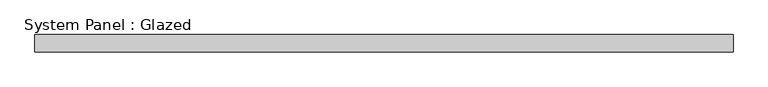
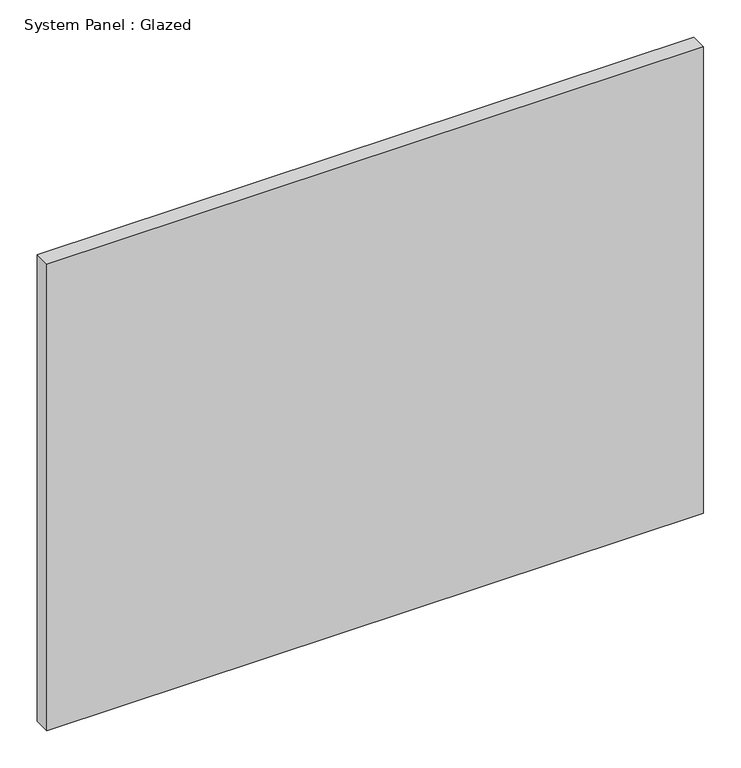
"""IFC4 building model written with IfcOpenShell, lengths in millimetres: plate geometry, System Panel : Glazed."""

from ifc_helpers import new_model, si_unit, origin, origin_with_axes, place, context, project, spatial, polyline, outline, extrude, source, transform, mapped, element, save


def system_panel_glazed_51d5fa28(model_context):
    return source(origin(), model_context, "Body", "SweptSolid", [
        extrude(outline(polyline([(508.92075, 19.05), (-508.92075, 19.05), (-508.92075, 44.45), (508.92075, 44.45), (508.92075, 19.05)])), origin_with_axes(), (0.0, 0.0, 1.0), 763.8415),
    ])


if __name__ == "__main__":
    model = new_model("IFC4")
    model_context = context("Model", 3, world=origin())
    ifc_project = project(units=[si_unit("LENGTHUNIT", "METRE", prefix="MILLI")], contexts=[model_context])
    site = spatial("IfcSite", under=ifc_project)
    building = spatial("IfcBuilding", under=site)
    placement = place(None, origin())
    system_panel_glazed_shape = system_panel_glazed_51d5fa28(model_context)
    element("IfcPlate", 1, ObjectType="System Panel : Glazed", at=placement, inside=building, context=model_context, shape_type="MappedRepresentation", body=[
        mapped(system_panel_glazed_shape, transform((0.0, 0.0, 0.0), x_axis=(1.0, 0.0, 0.0), y_axis=(0.0, 1.0, 0.0), z_axis=(0.0, 0.0, 1.0))),
    ])
    save(model, "model.ifc")

# Revit data of these elements
# Type "System Panel : Glazed"
#   Construction Type Id = "GSP4R"
#   Analytic Construction = "1/8 in Pilkington single glazing"
#   Visual Light Transmittance = 0.9
#   Solar Heat Gain Coefficient = 0.86
#   Heat Transfer Coefficient (U) = 1.18115 BTU/(h·ft²·°F)
#   Define Thermal Properties by = 1
# Element 1 (IfcPlate, "System Panel : Glazed")
#   Materials on its faces: "Glass"
# Materials
#   "Glass": class "Glass", colour RGB 0 128 192, transparency 0.75, Description = "Soda Lime Glass", Cost = 0
